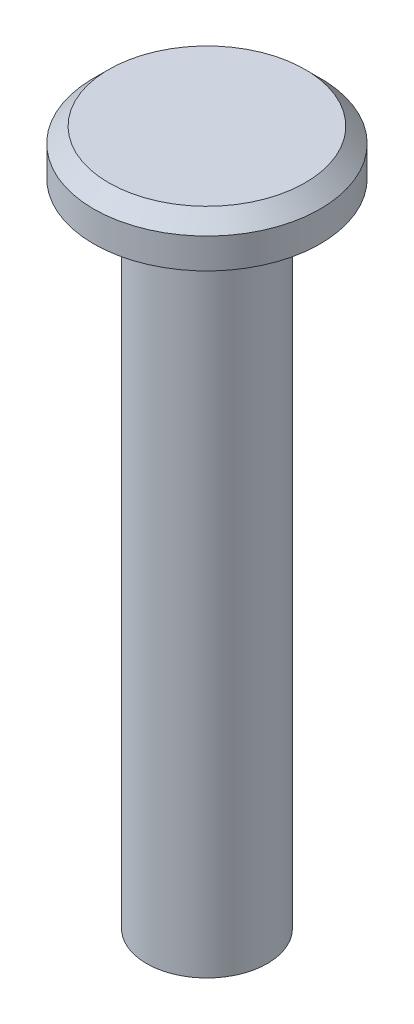
ISO-10303-21;
HEADER;
FILE_DESCRIPTION(('STEP AP214'),'2;1');
FILE_NAME('part.step','',(''),(''),'','','');
FILE_SCHEMA(('AUTOMOTIVE_DESIGN { 1 0 10303 214 1 1 1 1 }'));
ENDSEC;
DATA;
#1=APPLICATION_CONTEXT('core data for automotive mechanical design processes');
#2=APPLICATION_PROTOCOL_DEFINITION('international standard','automotive_design',2000,#1);
#3=PRODUCT_CONTEXT('',#1,'mechanical');
#4=PRODUCT('Part','Part','',(#3));
#5=PRODUCT_RELATED_PRODUCT_CATEGORY('part','',(#4));
#6=PRODUCT_DEFINITION_FORMATION('','',#4);
#7=PRODUCT_DEFINITION_CONTEXT('part definition',#1,'design');
#8=PRODUCT_DEFINITION('design','',#6,#7);
#9=PRODUCT_DEFINITION_SHAPE('','',#8);
#10=(LENGTH_UNIT() NAMED_UNIT(*) SI_UNIT(.MILLI.,.METRE.));
#11=(NAMED_UNIT(*) PLANE_ANGLE_UNIT() SI_UNIT($,.RADIAN.));
#12=(NAMED_UNIT(*) SI_UNIT($,.STERADIAN.) SOLID_ANGLE_UNIT());
#13=UNCERTAINTY_MEASURE_WITH_UNIT(LENGTH_MEASURE(1.E-05),#10,'distance_accuracy_value','');
#14=(GEOMETRIC_REPRESENTATION_CONTEXT(3) GLOBAL_UNCERTAINTY_ASSIGNED_CONTEXT((#13)) GLOBAL_UNIT_ASSIGNED_CONTEXT((#10,
#11,#12)) REPRESENTATION_CONTEXT('',''));
#15=CARTESIAN_POINT('',(0.,0.,0.));
#16=DIRECTION('',(0.,0.,1.));
#17=DIRECTION('',(1.,0.,0.));
#18=AXIS2_PLACEMENT_3D('',#15,#16,#17);
#19=CARTESIAN_POINT('',(0.,43.,0.));
#20=DIRECTION('',(0.,-1.,0.));
#21=DIRECTION('',(0.,0.,-1.));
#22=AXIS2_PLACEMENT_3D('',#19,#20,#21);
#23=CYLINDRICAL_SURFACE('',#22,4.);
#24=CARTESIAN_POINT('',(0.,43.,0.));
#25=DIRECTION('',(0.,1.,0.));
#26=DIRECTION('',(0.,0.,1.));
#27=AXIS2_PLACEMENT_3D('',#24,#25,#26);
#28=CIRCLE('',#27,4.);
#29=CARTESIAN_POINT('',(0.,43.,4.));
#30=VERTEX_POINT('',#29);
#31=EDGE_CURVE('E52',#30,#30,#28,.T.);
#32=ORIENTED_EDGE('',*,*,#31,.F.);
#33=EDGE_LOOP('',(#32));
#34=FACE_BOUND('',#33,.T.);
#35=CARTESIAN_POINT('',(0.,0.,0.));
#36=DIRECTION('',(0.,1.,0.));
#37=DIRECTION('',(0.,0.,1.));
#38=AXIS2_PLACEMENT_3D('',#35,#36,#37);
#39=CIRCLE('',#38,4.);
#40=CARTESIAN_POINT('',(0.,0.,4.));
#41=VERTEX_POINT('',#40);
#42=EDGE_CURVE('E60',#41,#41,#39,.T.);
#43=ORIENTED_EDGE('',*,*,#42,.T.);
#44=EDGE_LOOP('',(#43));
#45=FACE_BOUND('',#44,.T.);
#46=ADVANCED_FACE('F41',(#34,#45),#23,.T.);
#47=CARTESIAN_POINT('',(0.,0.,0.));
#48=DIRECTION('',(0.,1.,0.));
#49=DIRECTION('',(0.,0.,1.));
#50=AXIS2_PLACEMENT_3D('',#47,#48,#49);
#51=PLANE('',#50);
#52=ORIENTED_EDGE('',*,*,#42,.F.);
#53=EDGE_LOOP('',(#52));
#54=FACE_BOUND('',#53,.T.);
#55=ADVANCED_FACE('F81',(#54),#51,.F.);
#56=CARTESIAN_POINT('',(0.,46.,0.));
#57=DIRECTION('',(0.,-1.,0.));
#58=DIRECTION('',(0.,0.,-1.));
#59=AXIS2_PLACEMENT_3D('',#56,#57,#58);
#60=CYLINDRICAL_SURFACE('',#59,7.5);
#61=CARTESIAN_POINT('',(0.,45.,0.));
#62=DIRECTION('',(0.,1.,0.));
#63=DIRECTION('',(0.,0.,1.));
#64=AXIS2_PLACEMENT_3D('',#61,#62,#63);
#65=CIRCLE('',#64,7.5);
#66=CARTESIAN_POINT('',(0.,45.,7.5));
#67=VERTEX_POINT('',#66);
#68=EDGE_CURVE('E10',#67,#67,#65,.F.);
#69=ORIENTED_EDGE('',*,*,#68,.T.);
#70=EDGE_LOOP('',(#69));
#71=FACE_BOUND('',#70,.T.);
#72=CARTESIAN_POINT('',(0.,43.,0.));
#73=DIRECTION('',(0.,1.,0.));
#74=DIRECTION('',(0.,0.,1.));
#75=AXIS2_PLACEMENT_3D('',#72,#73,#74);
#76=CIRCLE('',#75,7.5);
#77=CARTESIAN_POINT('',(0.,43.,7.5));
#78=VERTEX_POINT('',#77);
#79=EDGE_CURVE('E61',#78,#78,#76,.T.);
#80=ORIENTED_EDGE('',*,*,#79,.T.);
#81=EDGE_LOOP('',(#80));
#82=FACE_BOUND('',#81,.T.);
#83=ADVANCED_FACE('F68',(#71,#82),#60,.T.);
#84=CARTESIAN_POINT('',(0.,46.,0.));
#85=DIRECTION('',(0.,1.,0.));
#86=DIRECTION('',(0.,0.,1.));
#87=AXIS2_PLACEMENT_3D('',#84,#85,#86);
#88=PLANE('',#87);
#89=CARTESIAN_POINT('',(0.,46.,0.));
#90=DIRECTION('',(0.,1.,0.));
#91=DIRECTION('',(0.,0.,1.));
#92=AXIS2_PLACEMENT_3D('',#89,#90,#91);
#93=CIRCLE('',#92,6.49999999999999);
#94=CARTESIAN_POINT('',(0.,46.,6.49999999999999));
#95=VERTEX_POINT('',#94);
#96=EDGE_CURVE('E47',#95,#95,#93,.T.);
#97=ORIENTED_EDGE('',*,*,#96,.T.);
#98=EDGE_LOOP('',(#97));
#99=FACE_BOUND('',#98,.T.);
#100=ADVANCED_FACE('F67',(#99),#88,.T.);
#101=CARTESIAN_POINT('',(0.,43.,0.));
#102=DIRECTION('',(0.,1.,0.));
#103=DIRECTION('',(0.,0.,1.));
#104=AXIS2_PLACEMENT_3D('',#101,#102,#103);
#105=PLANE('',#104);
#106=ORIENTED_EDGE('',*,*,#31,.T.);
#107=EDGE_LOOP('',(#106));
#108=FACE_BOUND('',#107,.T.);
#109=ORIENTED_EDGE('',*,*,#79,.F.);
#110=EDGE_LOOP('',(#109));
#111=FACE_BOUND('',#110,.T.);
#112=ADVANCED_FACE('F66',(#108,#111),#105,.F.);
#113=CARTESIAN_POINT('',(0.,46.,0.));
#114=DIRECTION('',(0.,-1.,0.));
#115=DIRECTION('',(0.,0.,-1.));
#116=AXIS2_PLACEMENT_3D('',#113,#114,#115);
#117=CONICAL_SURFACE('',#116,6.49999999999999,0.785398163397449);
#118=ORIENTED_EDGE('',*,*,#68,.F.);
#119=EDGE_LOOP('',(#118));
#120=FACE_BOUND('',#119,.T.);
#121=ORIENTED_EDGE('',*,*,#96,.F.);
#122=EDGE_LOOP('',(#121));
#123=FACE_BOUND('',#122,.T.);
#124=ADVANCED_FACE('F42',(#120,#123),#117,.T.);
#125=CLOSED_SHELL('',(#46,#55,#83,#100,#112,#124));
#126=MANIFOLD_SOLID_BREP('B2',#125);
#127=ADVANCED_BREP_SHAPE_REPRESENTATION('',(#18,#126),#14);
#128=SHAPE_DEFINITION_REPRESENTATION(#9,#127);
ENDSEC;
END-ISO-10303-21;
